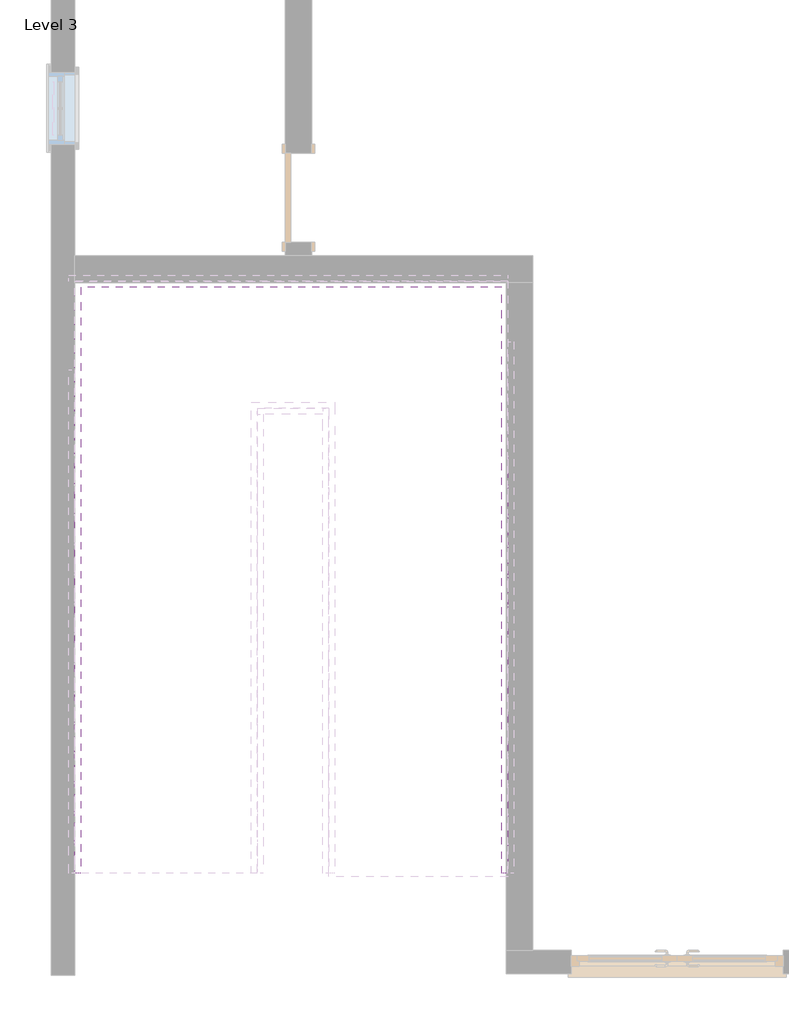
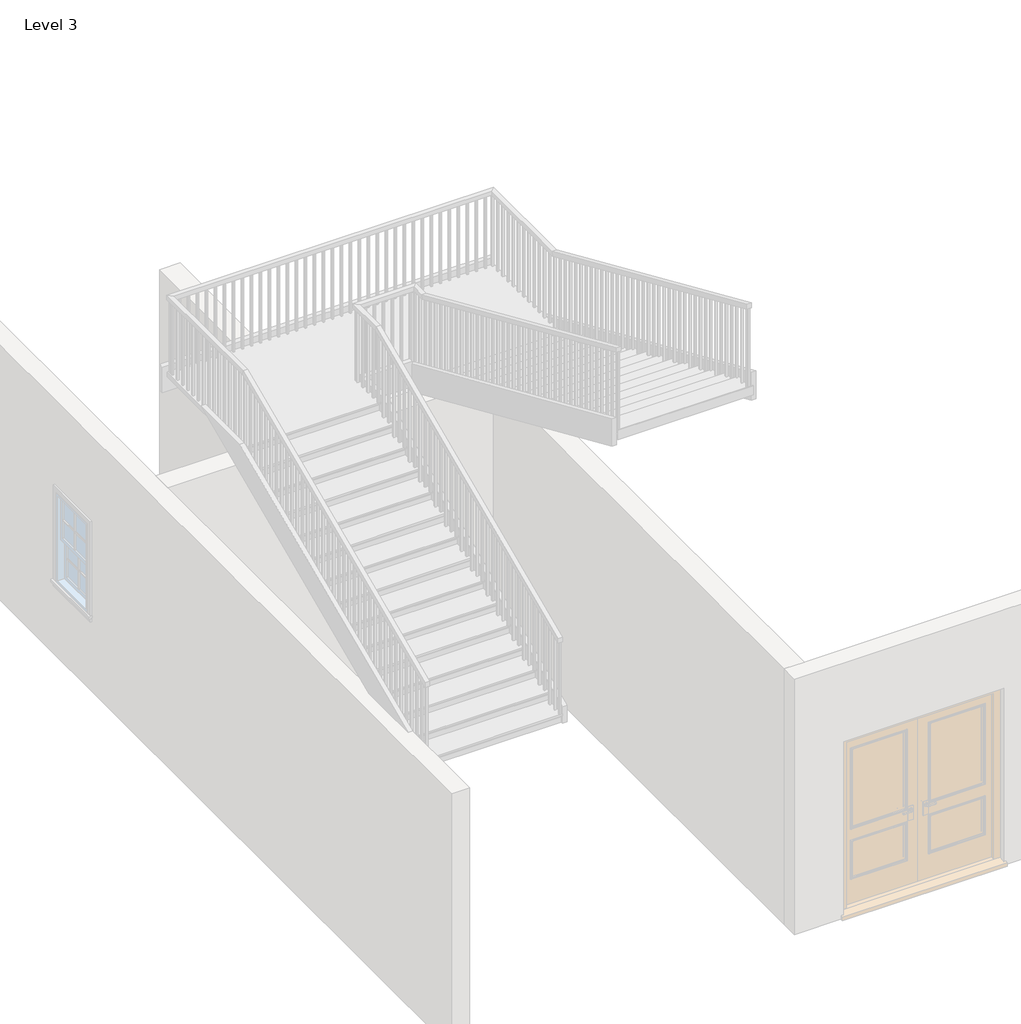
# One storey, part 5 of 6: 1 railing.
"""IFC4 building model written with IfcOpenShell, lengths in millimetres."""

from ifc_helpers import new_model, si_unit, frame, origin, place, context, project, spatial, polyline, outline, extrude, faceted_brep, element, save

model = new_model("IFC4")

# Units and contexts
model_context = context("Model", 3, world=origin())
ifc_project = project(units=[si_unit("LENGTHUNIT", "METRE", prefix="MILLI")], contexts=[model_context])

# Site, building, storey
site = spatial("IfcSite", under=ifc_project)
building = spatial("IfcBuilding", under=site)
storey = spatial("IfcBuildingStorey", under=building, Name="Level 3", Elevation=6096.0)

# Railing
placement = place(None, origin())
element("IfcRailing", 1, ObjectType="Handrail - Rectangular", at=placement, inside=storey, context=model_context, shape_type="SolidModel", body=[
    faceted_brep([(-7554.4415084, -6973.0610642, 9865.36), (-7554.4415084, -6973.0610642, 9809.8599828), (-7503.6415084, -6973.0610642, 9809.8599828), (-7503.6415084, -6973.0610642, 9865.36), (-7554.4415084, -3417.0610642, 11430.0), (-7554.4415084, -3406.3792071, 11379.2), (-7503.6415084, -3406.3792071, 11379.2), (-7503.6415084, -3417.0610642, 11430.0), (-7554.4415084, -1928.4217109, 11430.0), (-7554.4415084, -1928.4217109, 11379.2), (-7503.6415084, -1979.2217109, 11379.2), (-7503.6415084, -1979.2217109, 11430.0), (-3866.3290366, -1928.4217109, 11430.0), (-3866.3290366, -1928.4217109, 11379.2), (-3917.1290366, -1979.2217109, 11379.2), (-3917.1290366, -1979.2217109, 11430.0), (-3866.3290366, -3163.0610642, 11430.0), (-3866.3290366, -3173.7429214, 11379.2), (-3917.1290366, -3173.7429214, 11379.2), (-3917.1290366, -3163.0610642, 11430.0), (-3866.3290366, -6973.0610642, 13106.4), (-3917.1290366, -6973.0610642, 13106.4), (-3917.1290366, -6973.0610642, 13050.8999828), (-3866.3290366, -6973.0610642, 13050.8999828)], [[[0, 1, 2, 3]], [[1, 0, 4, 5]], [[2, 1, 5, 6]], [[3, 2, 6, 7]], [[0, 3, 7, 4]], [[5, 4, 8, 9]], [[6, 5, 9, 10]], [[7, 6, 10, 11]], [[4, 7, 11, 8]], [[9, 8, 12, 13]], [[10, 9, 13, 14]], [[11, 10, 14, 15]], [[8, 11, 15, 12]], [[13, 12, 16, 17]], [[14, 13, 17, 18]], [[15, 14, 18, 19]], [[12, 15, 19, 16]], [[20, 21, 22, 23]], [[17, 16, 20, 23]], [[18, 17, 23, 22]], [[19, 18, 22, 21]], [[16, 19, 21, 20]]]),
    extrude(outline(polyline([(-6922.6967109, 13028.7396674), (-6922.6967109, 12080.24), (-6941.7467109, 12080.24), (-6941.7467109, 13037.1216674), (-6922.6967109, 13028.7396674)])), frame((-3901.2540366, 0.0, 0.0), z_axis=(1.0, 0.0, 0.0), x_axis=(0.0, 1.0, 0.0)), (0.0, 0.0, 1.0), 19.05),
    extrude(outline(polyline([(-6821.0967109, 12984.0356674), (-6821.0967109, 12080.24), (-6840.1467109, 12080.24), (-6840.1467109, 12992.4176674), (-6821.0967109, 12984.0356674)])), frame((-3901.2540366, 0.0, 0.0), z_axis=(1.0, 0.0, 0.0), x_axis=(0.0, 1.0, 0.0)), (0.0, 0.0, 1.0), 19.05),
    extrude(outline(polyline([(-6719.4967109, 12939.3316674), (-6719.4967109, 12080.24), (-6738.5467109, 12080.24), (-6738.5467109, 12947.7136674), (-6719.4967109, 12939.3316674)])), frame((-3901.2540366, 0.0, 0.0), z_axis=(1.0, 0.0, 0.0), x_axis=(0.0, 1.0, 0.0)), (0.0, 0.0, 1.0), 19.05),
    extrude(outline(polyline([(-6617.8967109, 12894.6276674), (-6617.8967109, 11968.48), (-6636.9467109, 11968.48), (-6636.9467109, 12903.0096674), (-6617.8967109, 12894.6276674)])), frame((-3901.2540366, 0.0, 0.0), z_axis=(1.0, 0.0, 0.0), x_axis=(0.0, 1.0, 0.0)), (0.0, 0.0, 1.0), 19.05),
    extrude(outline(polyline([(-6516.2967109, 12849.9236674), (-6516.2967109, 11968.48), (-6535.3467109, 11968.48), (-6535.3467109, 12858.3056674), (-6516.2967109, 12849.9236674)])), frame((-3901.2540366, 0.0, 0.0), z_axis=(1.0, 0.0, 0.0), x_axis=(0.0, 1.0, 0.0)), (0.0, 0.0, 1.0), 19.05),
    extrude(outline(polyline([(-6414.6967109, 12805.2196674), (-6414.6967109, 11856.72), (-6433.7467109, 11856.72), (-6433.7467109, 12813.6016674), (-6414.6967109, 12805.2196674)])), frame((-3901.2540366, 0.0, 0.0), z_axis=(1.0, 0.0, 0.0), x_axis=(0.0, 1.0, 0.0)), (0.0, 0.0, 1.0), 19.05),
    extrude(outline(polyline([(-6313.0967109, 12760.5156674), (-6313.0967109, 11856.72), (-6332.1467109, 11856.72), (-6332.1467109, 12768.8976674), (-6313.0967109, 12760.5156674)])), frame((-3901.2540366, 0.0, 0.0), z_axis=(1.0, 0.0, 0.0), x_axis=(0.0, 1.0, 0.0)), (0.0, 0.0, 1.0), 19.05),
    extrude(outline(polyline([(-6211.4967109, 12715.8116674), (-6211.4967109, 11856.72), (-6230.5467109, 11856.72), (-6230.5467109, 12724.1936674), (-6211.4967109, 12715.8116674)])), frame((-3901.2540366, 0.0, 0.0), z_axis=(1.0, 0.0, 0.0), x_axis=(0.0, 1.0, 0.0)), (0.0, 0.0, 1.0), 19.05),
    extrude(outline(polyline([(-6109.8967109, 12671.1076674), (-6109.8967109, 11744.96), (-6128.9467109, 11744.96), (-6128.9467109, 12679.4896674), (-6109.8967109, 12671.1076674)])), frame((-3901.2540366, 0.0, 0.0), z_axis=(1.0, 0.0, 0.0), x_axis=(0.0, 1.0, 0.0)), (0.0, 0.0, 1.0), 19.05),
    extrude(outline(polyline([(-6008.2967109, 12626.4036674), (-6008.2967109, 11744.96), (-6027.3467109, 11744.96), (-6027.3467109, 12634.7856674), (-6008.2967109, 12626.4036674)])), frame((-3901.2540366, 0.0, 0.0), z_axis=(1.0, 0.0, 0.0), x_axis=(0.0, 1.0, 0.0)), (0.0, 0.0, 1.0), 19.05),
    extrude(outline(polyline([(-5906.6967109, 12581.6996674), (-5906.6967109, 11633.2), (-5925.7467109, 11633.2), (-5925.7467109, 12590.0816674), (-5906.6967109, 12581.6996674)])), frame((-3901.2540366, 0.0, 0.0), z_axis=(1.0, 0.0, 0.0), x_axis=(0.0, 1.0, 0.0)), (0.0, 0.0, 1.0), 19.05),
    extrude(outline(polyline([(-5805.0967109, 12536.9956674), (-5805.0967109, 11633.2), (-5824.1467109, 11633.2), (-5824.1467109, 12545.3776674), (-5805.0967109, 12536.9956674)])), frame((-3901.2540366, 0.0, 0.0), z_axis=(1.0, 0.0, 0.0), x_axis=(0.0, 1.0, 0.0)), (0.0, 0.0, 1.0), 19.05),
    extrude(outline(polyline([(-5703.4967109, 12492.2916674), (-5703.4967109, 11633.2), (-5722.5467109, 11633.2), (-5722.5467109, 12500.6736674), (-5703.4967109, 12492.2916674)])), frame((-3901.2540366, 0.0, 0.0), z_axis=(1.0, 0.0, 0.0), x_axis=(0.0, 1.0, 0.0)), (0.0, 0.0, 1.0), 19.05),
    extrude(outline(polyline([(-5601.8967109, 12447.5876674), (-5601.8967109, 11521.44), (-5620.9467109, 11521.44), (-5620.9467109, 12455.9696674), (-5601.8967109, 12447.5876674)])), frame((-3901.2540366, 0.0, 0.0), z_axis=(1.0, 0.0, 0.0), x_axis=(0.0, 1.0, 0.0)), (0.0, 0.0, 1.0), 19.05),
    extrude(outline(polyline([(-5500.2967109, 12402.8836674), (-5500.2967109, 11521.44), (-5519.3467109, 11521.44), (-5519.3467109, 12411.2656674), (-5500.2967109, 12402.8836674)])), frame((-3901.2540366, 0.0, 0.0), z_axis=(1.0, 0.0, 0.0), x_axis=(0.0, 1.0, 0.0)), (0.0, 0.0, 1.0), 19.05),
    extrude(outline(polyline([(-5398.6967109, 12358.1796674), (-5398.6967109, 11409.68), (-5417.7467109, 11409.68), (-5417.7467109, 12366.5616674), (-5398.6967109, 12358.1796674)])), frame((-3901.2540366, 0.0, 0.0), z_axis=(1.0, 0.0, 0.0), x_axis=(0.0, 1.0, 0.0)), (0.0, 0.0, 1.0), 19.05),
    extrude(outline(polyline([(-5297.0967109, 12313.4756674), (-5297.0967109, 11409.68), (-5316.1467109, 11409.68), (-5316.1467109, 12321.8576674), (-5297.0967109, 12313.4756674)])), frame((-3901.2540366, 0.0, 0.0), z_axis=(1.0, 0.0, 0.0), x_axis=(0.0, 1.0, 0.0)), (0.0, 0.0, 1.0), 19.05),
    extrude(outline(polyline([(-5195.4967109, 12268.7716674), (-5195.4967109, 11409.68), (-5214.5467109, 11409.68), (-5214.5467109, 12277.1536674), (-5195.4967109, 12268.7716674)])), frame((-3901.2540366, 0.0, 0.0), z_axis=(1.0, 0.0, 0.0), x_axis=(0.0, 1.0, 0.0)), (0.0, 0.0, 1.0), 19.05),
    extrude(outline(polyline([(-5093.8967109, 12224.0676674), (-5093.8967109, 11297.92), (-5112.9467109, 11297.92), (-5112.9467109, 12232.4496674), (-5093.8967109, 12224.0676674)])), frame((-3901.2540366, 0.0, 0.0), z_axis=(1.0, 0.0, 0.0), x_axis=(0.0, 1.0, 0.0)), (0.0, 0.0, 1.0), 19.05),
    extrude(outline(polyline([(-4992.2967109, 12179.3636674), (-4992.2967109, 11297.92), (-5011.3467109, 11297.92), (-5011.3467109, 12187.7456674), (-4992.2967109, 12179.3636674)])), frame((-3901.2540366, 0.0, 0.0), z_axis=(1.0, 0.0, 0.0), x_axis=(0.0, 1.0, 0.0)), (0.0, 0.0, 1.0), 19.05),
    extrude(outline(polyline([(-4890.6967109, 12134.6596674), (-4890.6967109, 11186.16), (-4909.7467109, 11186.16), (-4909.7467109, 12143.0416674), (-4890.6967109, 12134.6596674)])), frame((-3901.2540366, 0.0, 0.0), z_axis=(1.0, 0.0, 0.0), x_axis=(0.0, 1.0, 0.0)), (0.0, 0.0, 1.0), 19.05),
    extrude(outline(polyline([(-4789.0967109, 12089.9556674), (-4789.0967109, 11186.16), (-4808.1467109, 11186.16), (-4808.1467109, 12098.3376674), (-4789.0967109, 12089.9556674)])), frame((-3901.2540366, 0.0, 0.0), z_axis=(1.0, 0.0, 0.0), x_axis=(0.0, 1.0, 0.0)), (0.0, 0.0, 1.0), 19.05),
    extrude(outline(polyline([(-4687.4967109, 12045.2516674), (-4687.4967109, 11186.16), (-4706.5467109, 11186.16), (-4706.5467109, 12053.6336674), (-4687.4967109, 12045.2516674)])), frame((-3901.2540366, 0.0, 0.0), z_axis=(1.0, 0.0, 0.0), x_axis=(0.0, 1.0, 0.0)), (0.0, 0.0, 1.0), 19.05),
    extrude(outline(polyline([(-4585.8967109, 12000.5476674), (-4585.8967109, 11074.4), (-4604.9467109, 11074.4), (-4604.9467109, 12008.9296674), (-4585.8967109, 12000.5476674)])), frame((-3901.2540366, 0.0, 0.0), z_axis=(1.0, 0.0, 0.0), x_axis=(0.0, 1.0, 0.0)), (0.0, 0.0, 1.0), 19.05),
    extrude(outline(polyline([(-4484.2967109, 11955.8436674), (-4484.2967109, 11074.4), (-4503.3467109, 11074.4), (-4503.3467109, 11964.2256674), (-4484.2967109, 11955.8436674)])), frame((-3901.2540366, 0.0, 0.0), z_axis=(1.0, 0.0, 0.0), x_axis=(0.0, 1.0, 0.0)), (0.0, 0.0, 1.0), 19.05),
    extrude(outline(polyline([(-4382.6967109, 11911.1396674), (-4382.6967109, 10962.64), (-4401.7467109, 10962.64), (-4401.7467109, 11919.5216674), (-4382.6967109, 11911.1396674)])), frame((-3901.2540366, 0.0, 0.0), z_axis=(1.0, 0.0, 0.0), x_axis=(0.0, 1.0, 0.0)), (0.0, 0.0, 1.0), 19.05),
    extrude(outline(polyline([(-4281.0967109, 11866.4356674), (-4281.0967109, 10962.64), (-4300.1467109, 10962.64), (-4300.1467109, 11874.8176674), (-4281.0967109, 11866.4356674)])), frame((-3901.2540366, 0.0, 0.0), z_axis=(1.0, 0.0, 0.0), x_axis=(0.0, 1.0, 0.0)), (0.0, 0.0, 1.0), 19.05),
    extrude(outline(polyline([(-4179.4967109, 11821.7316674), (-4179.4967109, 10962.64), (-4198.5467109, 10962.64), (-4198.5467109, 11830.1136674), (-4179.4967109, 11821.7316674)])), frame((-3901.2540366, 0.0, 0.0), z_axis=(1.0, 0.0, 0.0), x_axis=(0.0, 1.0, 0.0)), (0.0, 0.0, 1.0), 19.05),
    extrude(outline(polyline([(-4077.8967109, 11777.0276674), (-4077.8967109, 10850.88), (-4096.9467109, 10850.88), (-4096.9467109, 11785.4096674), (-4077.8967109, 11777.0276674)])), frame((-3901.2540366, 0.0, 0.0), z_axis=(1.0, 0.0, 0.0), x_axis=(0.0, 1.0, 0.0)), (0.0, 0.0, 1.0), 19.05),
    extrude(outline(polyline([(-3976.2967109, 11732.3236674), (-3976.2967109, 10850.88), (-3995.3467109, 10850.88), (-3995.3467109, 11740.7056674), (-3976.2967109, 11732.3236674)])), frame((-3901.2540366, 0.0, 0.0), z_axis=(1.0, 0.0, 0.0), x_axis=(0.0, 1.0, 0.0)), (0.0, 0.0, 1.0), 19.05),
    extrude(outline(polyline([(-3874.6967109, 11687.6196674), (-3874.6967109, 10739.12), (-3893.7467109, 10739.12), (-3893.7467109, 11696.0016674), (-3874.6967109, 11687.6196674)])), frame((-3901.2540366, 0.0, 0.0), z_axis=(1.0, 0.0, 0.0), x_axis=(0.0, 1.0, 0.0)), (0.0, 0.0, 1.0), 19.05),
    extrude(outline(polyline([(-3773.0967109, 11642.9156674), (-3773.0967109, 10739.12), (-3792.1467109, 10739.12), (-3792.1467109, 11651.2976674), (-3773.0967109, 11642.9156674)])), frame((-3901.2540366, 0.0, 0.0), z_axis=(1.0, 0.0, 0.0), x_axis=(0.0, 1.0, 0.0)), (0.0, 0.0, 1.0), 19.05),
    extrude(outline(polyline([(-3671.4967109, 11598.2116674), (-3671.4967109, 10739.12), (-3690.5467109, 10739.12), (-3690.5467109, 11606.5936674), (-3671.4967109, 11598.2116674)])), frame((-3901.2540366, 0.0, 0.0), z_axis=(1.0, 0.0, 0.0), x_axis=(0.0, 1.0, 0.0)), (0.0, 0.0, 1.0), 19.05),
    extrude(outline(polyline([(-3569.8967109, 11553.5076674), (-3569.8967109, 10627.36), (-3588.9467109, 10627.36), (-3588.9467109, 11561.8896674), (-3569.8967109, 11553.5076674)])), frame((-3901.2540366, 0.0, 0.0), z_axis=(1.0, 0.0, 0.0), x_axis=(0.0, 1.0, 0.0)), (0.0, 0.0, 1.0), 19.05),
    extrude(outline(polyline([(-3468.2967109, 11508.8036674), (-3468.2967109, 10627.36), (-3487.3467109, 10627.36), (-3487.3467109, 11517.1856674), (-3468.2967109, 11508.8036674)])), frame((-3901.2540366, 0.0, 0.0), z_axis=(1.0, 0.0, 0.0), x_axis=(0.0, 1.0, 0.0)), (0.0, 0.0, 1.0), 19.05),
    extrude(outline(polyline([(-3366.6967109, 11464.0996674), (-3366.6967109, 10515.6), (-3385.7467109, 10515.6), (-3385.7467109, 11472.4816674), (-3366.6967109, 11464.0996674)])), frame((-3901.2540366, 0.0, 0.0), z_axis=(1.0, 0.0, 0.0), x_axis=(0.0, 1.0, 0.0)), (0.0, 0.0, 1.0), 19.05),
    extrude(outline(polyline([(-3265.0967109, 11419.3956674), (-3265.0967109, 10515.6), (-3284.1467109, 10515.6), (-3284.1467109, 11427.7776674), (-3265.0967109, 11419.3956674)])), frame((-3901.2540366, 0.0, 0.0), z_axis=(1.0, 0.0, 0.0), x_axis=(0.0, 1.0, 0.0)), (0.0, 0.0, 1.0), 19.05),
    extrude(outline(polyline([(-3163.4967109, 11374.6916674), (-3163.4967109, 10515.6), (-3182.5467109, 10515.6), (-3182.5467109, 11383.0736674), (-3163.4967109, 11374.6916674)])), frame((-3901.2540366, 0.0, 0.0), z_axis=(1.0, 0.0, 0.0), x_axis=(0.0, 1.0, 0.0)), (0.0, 0.0, 1.0), 19.05),
    extrude(outline(polyline([(-3882.2040366, -3061.8967109), (-3882.2040366, -3080.9467109), (-3901.2540366, -3080.9467109), (-3901.2540366, -3061.8967109), (-3882.2040366, -3061.8967109)])), frame((0.0, 0.0, 10515.6), z_axis=(0.0, 0.0, 1.0), x_axis=(1.0, 0.0, 0.0)), (0.0, 0.0, 1.0), 863.6),
    extrude(outline(polyline([(-3882.2040366, -2960.2967109), (-3882.2040366, -2979.3467109), (-3901.2540366, -2979.3467109), (-3901.2540366, -2960.2967109), (-3882.2040366, -2960.2967109)])), frame((0.0, 0.0, 10515.6), z_axis=(0.0, 0.0, 1.0), x_axis=(1.0, 0.0, 0.0)), (0.0, 0.0, 1.0), 863.6),
    extrude(outline(polyline([(-3882.2040366, -2858.6967109), (-3882.2040366, -2877.7467109), (-3901.2540366, -2877.7467109), (-3901.2540366, -2858.6967109), (-3882.2040366, -2858.6967109)])), frame((0.0, 0.0, 10515.6), z_axis=(0.0, 0.0, 1.0), x_axis=(1.0, 0.0, 0.0)), (0.0, 0.0, 1.0), 863.6),
    extrude(outline(polyline([(-3882.2040366, -2757.0967109), (-3882.2040366, -2776.1467109), (-3901.2540366, -2776.1467109), (-3901.2540366, -2757.0967109), (-3882.2040366, -2757.0967109)])), frame((0.0, 0.0, 10515.6), z_axis=(0.0, 0.0, 1.0), x_axis=(1.0, 0.0, 0.0)), (0.0, 0.0, 1.0), 863.6),
    extrude(outline(polyline([(-3882.2040366, -2655.4967109), (-3882.2040366, -2674.5467109), (-3901.2540366, -2674.5467109), (-3901.2540366, -2655.4967109), (-3882.2040366, -2655.4967109)])), frame((0.0, 0.0, 10515.6), z_axis=(0.0, 0.0, 1.0), x_axis=(1.0, 0.0, 0.0)), (0.0, 0.0, 1.0), 863.6),
    extrude(outline(polyline([(-3882.2040366, -2553.8967109), (-3882.2040366, -2572.9467109), (-3901.2540366, -2572.9467109), (-3901.2540366, -2553.8967109), (-3882.2040366, -2553.8967109)])), frame((0.0, 0.0, 10515.6), z_axis=(0.0, 0.0, 1.0), x_axis=(1.0, 0.0, 0.0)), (0.0, 0.0, 1.0), 863.6),
    extrude(outline(polyline([(-3882.2040366, -2452.2967109), (-3882.2040366, -2471.3467109), (-3901.2540366, -2471.3467109), (-3901.2540366, -2452.2967109), (-3882.2040366, -2452.2967109)])), frame((0.0, 0.0, 10515.6), z_axis=(0.0, 0.0, 1.0), x_axis=(1.0, 0.0, 0.0)), (0.0, 0.0, 1.0), 863.6),
    extrude(outline(polyline([(-3882.2040366, -2350.6967109), (-3882.2040366, -2369.7467109), (-3901.2540366, -2369.7467109), (-3901.2540366, -2350.6967109), (-3882.2040366, -2350.6967109)])), frame((0.0, 0.0, 10515.6), z_axis=(0.0, 0.0, 1.0), x_axis=(1.0, 0.0, 0.0)), (0.0, 0.0, 1.0), 863.6),
    extrude(outline(polyline([(-3882.2040366, -2249.0967109), (-3882.2040366, -2268.1467109), (-3901.2540366, -2268.1467109), (-3901.2540366, -2249.0967109), (-3882.2040366, -2249.0967109)])), frame((0.0, 0.0, 10515.6), z_axis=(0.0, 0.0, 1.0), x_axis=(1.0, 0.0, 0.0)), (0.0, 0.0, 1.0), 863.6),
    extrude(outline(polyline([(-3882.2040366, -2147.4967109), (-3882.2040366, -2166.5467109), (-3901.2540366, -2166.5467109), (-3901.2540366, -2147.4967109), (-3882.2040366, -2147.4967109)])), frame((0.0, 0.0, 10515.6), z_axis=(0.0, 0.0, 1.0), x_axis=(1.0, 0.0, 0.0)), (0.0, 0.0, 1.0), 863.6),
    extrude(outline(polyline([(-3882.2040366, -2045.8967109), (-3882.2040366, -2064.9467109), (-3901.2540366, -2064.9467109), (-3901.2540366, -2045.8967109), (-3882.2040366, -2045.8967109)])), frame((0.0, 0.0, 10515.6), z_axis=(0.0, 0.0, 1.0), x_axis=(1.0, 0.0, 0.0)), (0.0, 0.0, 1.0), 863.6),
    extrude(outline(polyline([(-3982.5665084, -1944.2967109), (-3963.5165084, -1944.2967109), (-3963.5165084, -1963.3467109), (-3982.5665084, -1963.3467109), (-3982.5665084, -1944.2967109)])), frame((0.0, 0.0, 10515.6), z_axis=(0.0, 0.0, 1.0), x_axis=(1.0, 0.0, 0.0)), (0.0, 0.0, 1.0), 863.6),
    extrude(outline(polyline([(-4084.1665084, -1944.2967109), (-4065.1165084, -1944.2967109), (-4065.1165084, -1963.3467109), (-4084.1665084, -1963.3467109), (-4084.1665084, -1944.2967109)])), frame((0.0, 0.0, 10515.6), z_axis=(0.0, 0.0, 1.0), x_axis=(1.0, 0.0, 0.0)), (0.0, 0.0, 1.0), 863.6),
    extrude(outline(polyline([(-4185.7665084, -1944.2967109), (-4166.7165084, -1944.2967109), (-4166.7165084, -1963.3467109), (-4185.7665084, -1963.3467109), (-4185.7665084, -1944.2967109)])), frame((0.0, 0.0, 10515.6), z_axis=(0.0, 0.0, 1.0), x_axis=(1.0, 0.0, 0.0)), (0.0, 0.0, 1.0), 863.6),
    extrude(outline(polyline([(-4287.3665084, -1944.2967109), (-4268.3165084, -1944.2967109), (-4268.3165084, -1963.3467109), (-4287.3665084, -1963.3467109), (-4287.3665084, -1944.2967109)])), frame((0.0, 0.0, 10515.6), z_axis=(0.0, 0.0, 1.0), x_axis=(1.0, 0.0, 0.0)), (0.0, 0.0, 1.0), 863.6),
    extrude(outline(polyline([(-4388.9665084, -1944.2967109), (-4369.9165084, -1944.2967109), (-4369.9165084, -1963.3467109), (-4388.9665084, -1963.3467109), (-4388.9665084, -1944.2967109)])), frame((0.0, 0.0, 10515.6), z_axis=(0.0, 0.0, 1.0), x_axis=(1.0, 0.0, 0.0)), (0.0, 0.0, 1.0), 863.6),
    extrude(outline(polyline([(-4490.5665084, -1944.2967109), (-4471.5165084, -1944.2967109), (-4471.5165084, -1963.3467109), (-4490.5665084, -1963.3467109), (-4490.5665084, -1944.2967109)])), frame((0.0, 0.0, 10515.6), z_axis=(0.0, 0.0, 1.0), x_axis=(1.0, 0.0, 0.0)), (0.0, 0.0, 1.0), 863.6),
    extrude(outline(polyline([(-4592.1665084, -1944.2967109), (-4573.1165084, -1944.2967109), (-4573.1165084, -1963.3467109), (-4592.1665084, -1963.3467109), (-4592.1665084, -1944.2967109)])), frame((0.0, 0.0, 10515.6), z_axis=(0.0, 0.0, 1.0), x_axis=(1.0, 0.0, 0.0)), (0.0, 0.0, 1.0), 863.6),
    extrude(outline(polyline([(-4693.7665084, -1944.2967109), (-4674.7165084, -1944.2967109), (-4674.7165084, -1963.3467109), (-4693.7665084, -1963.3467109), (-4693.7665084, -1944.2967109)])), frame((0.0, 0.0, 10515.6), z_axis=(0.0, 0.0, 1.0), x_axis=(1.0, 0.0, 0.0)), (0.0, 0.0, 1.0), 863.6),
    extrude(outline(polyline([(-4795.3665084, -1944.2967109), (-4776.3165084, -1944.2967109), (-4776.3165084, -1963.3467109), (-4795.3665084, -1963.3467109), (-4795.3665084, -1944.2967109)])), frame((0.0, 0.0, 10515.6), z_axis=(0.0, 0.0, 1.0), x_axis=(1.0, 0.0, 0.0)), (0.0, 0.0, 1.0), 863.6),
    extrude(outline(polyline([(-4896.9665084, -1944.2967109), (-4877.9165084, -1944.2967109), (-4877.9165084, -1963.3467109), (-4896.9665084, -1963.3467109), (-4896.9665084, -1944.2967109)])), frame((0.0, 0.0, 10515.6), z_axis=(0.0, 0.0, 1.0), x_axis=(1.0, 0.0, 0.0)), (0.0, 0.0, 1.0), 863.6),
    extrude(outline(polyline([(-4998.5665084, -1944.2967109), (-4979.5165084, -1944.2967109), (-4979.5165084, -1963.3467109), (-4998.5665084, -1963.3467109), (-4998.5665084, -1944.2967109)])), frame((0.0, 0.0, 10515.6), z_axis=(0.0, 0.0, 1.0), x_axis=(1.0, 0.0, 0.0)), (0.0, 0.0, 1.0), 863.6),
    extrude(outline(polyline([(-5100.1665084, -1944.2967109), (-5081.1165084, -1944.2967109), (-5081.1165084, -1963.3467109), (-5100.1665084, -1963.3467109), (-5100.1665084, -1944.2967109)])), frame((0.0, 0.0, 10515.6), z_axis=(0.0, 0.0, 1.0), x_axis=(1.0, 0.0, 0.0)), (0.0, 0.0, 1.0), 863.6),
    extrude(outline(polyline([(-5201.7665084, -1944.2967109), (-5182.7165084, -1944.2967109), (-5182.7165084, -1963.3467109), (-5201.7665084, -1963.3467109), (-5201.7665084, -1944.2967109)])), frame((0.0, 0.0, 10515.6), z_axis=(0.0, 0.0, 1.0), x_axis=(1.0, 0.0, 0.0)), (0.0, 0.0, 1.0), 863.6),
    extrude(outline(polyline([(-5303.3665084, -1944.2967109), (-5284.3165084, -1944.2967109), (-5284.3165084, -1963.3467109), (-5303.3665084, -1963.3467109), (-5303.3665084, -1944.2967109)])), frame((0.0, 0.0, 10515.6), z_axis=(0.0, 0.0, 1.0), x_axis=(1.0, 0.0, 0.0)), (0.0, 0.0, 1.0), 863.6),
    extrude(outline(polyline([(-5404.9665084, -1944.2967109), (-5385.9165084, -1944.2967109), (-5385.9165084, -1963.3467109), (-5404.9665084, -1963.3467109), (-5404.9665084, -1944.2967109)])), frame((0.0, 0.0, 10515.6), z_axis=(0.0, 0.0, 1.0), x_axis=(1.0, 0.0, 0.0)), (0.0, 0.0, 1.0), 863.6),
    extrude(outline(polyline([(-5506.5665084, -1944.2967109), (-5487.5165084, -1944.2967109), (-5487.5165084, -1963.3467109), (-5506.5665084, -1963.3467109), (-5506.5665084, -1944.2967109)])), frame((0.0, 0.0, 10515.6), z_axis=(0.0, 0.0, 1.0), x_axis=(1.0, 0.0, 0.0)), (0.0, 0.0, 1.0), 863.6),
    extrude(outline(polyline([(-5608.1665084, -1944.2967109), (-5589.1165084, -1944.2967109), (-5589.1165084, -1963.3467109), (-5608.1665084, -1963.3467109), (-5608.1665084, -1944.2967109)])), frame((0.0, 0.0, 10515.6), z_axis=(0.0, 0.0, 1.0), x_axis=(1.0, 0.0, 0.0)), (0.0, 0.0, 1.0), 863.6),
    extrude(outline(polyline([(-5709.7665084, -1944.2967109), (-5690.7165084, -1944.2967109), (-5690.7165084, -1963.3467109), (-5709.7665084, -1963.3467109), (-5709.7665084, -1944.2967109)])), frame((0.0, 0.0, 10515.6), z_axis=(0.0, 0.0, 1.0), x_axis=(1.0, 0.0, 0.0)), (0.0, 0.0, 1.0), 863.6),
    extrude(outline(polyline([(-5811.3665084, -1944.2967109), (-5792.3165084, -1944.2967109), (-5792.3165084, -1963.3467109), (-5811.3665084, -1963.3467109), (-5811.3665084, -1944.2967109)])), frame((0.0, 0.0, 10515.6), z_axis=(0.0, 0.0, 1.0), x_axis=(1.0, 0.0, 0.0)), (0.0, 0.0, 1.0), 863.6),
    extrude(outline(polyline([(-5912.9665084, -1944.2967109), (-5893.9165084, -1944.2967109), (-5893.9165084, -1963.3467109), (-5912.9665084, -1963.3467109), (-5912.9665084, -1944.2967109)])), frame((0.0, 0.0, 10515.6), z_axis=(0.0, 0.0, 1.0), x_axis=(1.0, 0.0, 0.0)), (0.0, 0.0, 1.0), 863.6),
    extrude(outline(polyline([(-6014.5665084, -1944.2967109), (-5995.5165084, -1944.2967109), (-5995.5165084, -1963.3467109), (-6014.5665084, -1963.3467109), (-6014.5665084, -1944.2967109)])), frame((0.0, 0.0, 10515.6), z_axis=(0.0, 0.0, 1.0), x_axis=(1.0, 0.0, 0.0)), (0.0, 0.0, 1.0), 863.6),
    extrude(outline(polyline([(-6116.1665084, -1944.2967109), (-6097.1165084, -1944.2967109), (-6097.1165084, -1963.3467109), (-6116.1665084, -1963.3467109), (-6116.1665084, -1944.2967109)])), frame((0.0, 0.0, 10515.6), z_axis=(0.0, 0.0, 1.0), x_axis=(1.0, 0.0, 0.0)), (0.0, 0.0, 1.0), 863.6),
    extrude(outline(polyline([(-6217.7665084, -1944.2967109), (-6198.7165084, -1944.2967109), (-6198.7165084, -1963.3467109), (-6217.7665084, -1963.3467109), (-6217.7665084, -1944.2967109)])), frame((0.0, 0.0, 10515.6), z_axis=(0.0, 0.0, 1.0), x_axis=(1.0, 0.0, 0.0)), (0.0, 0.0, 1.0), 863.6),
    extrude(outline(polyline([(-6319.3665084, -1944.2967109), (-6300.3165084, -1944.2967109), (-6300.3165084, -1963.3467109), (-6319.3665084, -1963.3467109), (-6319.3665084, -1944.2967109)])), frame((0.0, 0.0, 10515.6), z_axis=(0.0, 0.0, 1.0), x_axis=(1.0, 0.0, 0.0)), (0.0, 0.0, 1.0), 863.6),
    extrude(outline(polyline([(-6420.9665084, -1944.2967109), (-6401.9165084, -1944.2967109), (-6401.9165084, -1963.3467109), (-6420.9665084, -1963.3467109), (-6420.9665084, -1944.2967109)])), frame((0.0, 0.0, 10515.6), z_axis=(0.0, 0.0, 1.0), x_axis=(1.0, 0.0, 0.0)), (0.0, 0.0, 1.0), 863.6),
    extrude(outline(polyline([(-6522.5665084, -1944.2967109), (-6503.5165084, -1944.2967109), (-6503.5165084, -1963.3467109), (-6522.5665084, -1963.3467109), (-6522.5665084, -1944.2967109)])), frame((0.0, 0.0, 10515.6), z_axis=(0.0, 0.0, 1.0), x_axis=(1.0, 0.0, 0.0)), (0.0, 0.0, 1.0), 863.6),
    extrude(outline(polyline([(-6624.1665084, -1944.2967109), (-6605.1165084, -1944.2967109), (-6605.1165084, -1963.3467109), (-6624.1665084, -1963.3467109), (-6624.1665084, -1944.2967109)])), frame((0.0, 0.0, 10515.6), z_axis=(0.0, 0.0, 1.0), x_axis=(1.0, 0.0, 0.0)), (0.0, 0.0, 1.0), 863.6),
    extrude(outline(polyline([(-6725.7665084, -1944.2967109), (-6706.7165084, -1944.2967109), (-6706.7165084, -1963.3467109), (-6725.7665084, -1963.3467109), (-6725.7665084, -1944.2967109)])), frame((0.0, 0.0, 10515.6), z_axis=(0.0, 0.0, 1.0), x_axis=(1.0, 0.0, 0.0)), (0.0, 0.0, 1.0), 863.6),
    extrude(outline(polyline([(-6827.3665084, -1944.2967109), (-6808.3165084, -1944.2967109), (-6808.3165084, -1963.3467109), (-6827.3665084, -1963.3467109), (-6827.3665084, -1944.2967109)])), frame((0.0, 0.0, 10515.6), z_axis=(0.0, 0.0, 1.0), x_axis=(1.0, 0.0, 0.0)), (0.0, 0.0, 1.0), 863.6),
    extrude(outline(polyline([(-6928.9665084, -1944.2967109), (-6909.9165084, -1944.2967109), (-6909.9165084, -1963.3467109), (-6928.9665084, -1963.3467109), (-6928.9665084, -1944.2967109)])), frame((0.0, 0.0, 10515.6), z_axis=(0.0, 0.0, 1.0), x_axis=(1.0, 0.0, 0.0)), (0.0, 0.0, 1.0), 863.6),
    extrude(outline(polyline([(-7030.5665084, -1944.2967109), (-7011.5165084, -1944.2967109), (-7011.5165084, -1963.3467109), (-7030.5665084, -1963.3467109), (-7030.5665084, -1944.2967109)])), frame((0.0, 0.0, 10515.6), z_axis=(0.0, 0.0, 1.0), x_axis=(1.0, 0.0, 0.0)), (0.0, 0.0, 1.0), 863.6),
    extrude(outline(polyline([(-7132.1665084, -1944.2967109), (-7113.1165084, -1944.2967109), (-7113.1165084, -1963.3467109), (-7132.1665084, -1963.3467109), (-7132.1665084, -1944.2967109)])), frame((0.0, 0.0, 10515.6), z_axis=(0.0, 0.0, 1.0), x_axis=(1.0, 0.0, 0.0)), (0.0, 0.0, 1.0), 863.6),
    extrude(outline(polyline([(-7233.7665084, -1944.2967109), (-7214.7165084, -1944.2967109), (-7214.7165084, -1963.3467109), (-7233.7665084, -1963.3467109), (-7233.7665084, -1944.2967109)])), frame((0.0, 0.0, 10515.6), z_axis=(0.0, 0.0, 1.0), x_axis=(1.0, 0.0, 0.0)), (0.0, 0.0, 1.0), 863.6),
    extrude(outline(polyline([(-7335.3665084, -1944.2967109), (-7316.3165084, -1944.2967109), (-7316.3165084, -1963.3467109), (-7335.3665084, -1963.3467109), (-7335.3665084, -1944.2967109)])), frame((0.0, 0.0, 10515.6), z_axis=(0.0, 0.0, 1.0), x_axis=(1.0, 0.0, 0.0)), (0.0, 0.0, 1.0), 863.6),
    extrude(outline(polyline([(-7436.9665084, -1944.2967109), (-7417.9165084, -1944.2967109), (-7417.9165084, -1963.3467109), (-7436.9665084, -1963.3467109), (-7436.9665084, -1944.2967109)])), frame((0.0, 0.0, 10515.6), z_axis=(0.0, 0.0, 1.0), x_axis=(1.0, 0.0, 0.0)), (0.0, 0.0, 1.0), 863.6),
    extrude(outline(polyline([(-7538.5665084, -2004.1860642), (-7538.5665084, -1985.1360642), (-7519.5165084, -1985.1360642), (-7519.5165084, -2004.1860642), (-7538.5665084, -2004.1860642)])), frame((0.0, 0.0, 10515.6), z_axis=(0.0, 0.0, 1.0), x_axis=(1.0, 0.0, 0.0)), (0.0, 0.0, 1.0), 863.6),
    extrude(outline(polyline([(-7538.5665084, -2105.7860642), (-7538.5665084, -2086.7360642), (-7519.5165084, -2086.7360642), (-7519.5165084, -2105.7860642), (-7538.5665084, -2105.7860642)])), frame((0.0, 0.0, 10515.6), z_axis=(0.0, 0.0, 1.0), x_axis=(1.0, 0.0, 0.0)), (0.0, 0.0, 1.0), 863.6),
    extrude(outline(polyline([(-7538.5665084, -2207.3860642), (-7538.5665084, -2188.3360642), (-7519.5165084, -2188.3360642), (-7519.5165084, -2207.3860642), (-7538.5665084, -2207.3860642)])), frame((0.0, 0.0, 10515.6), z_axis=(0.0, 0.0, 1.0), x_axis=(1.0, 0.0, 0.0)), (0.0, 0.0, 1.0), 863.6),
    extrude(outline(polyline([(-7538.5665084, -2308.9860642), (-7538.5665084, -2289.9360642), (-7519.5165084, -2289.9360642), (-7519.5165084, -2308.9860642), (-7538.5665084, -2308.9860642)])), frame((0.0, 0.0, 10515.6), z_axis=(0.0, 0.0, 1.0), x_axis=(1.0, 0.0, 0.0)), (0.0, 0.0, 1.0), 863.6),
    extrude(outline(polyline([(-7538.5665084, -2410.5860642), (-7538.5665084, -2391.5360642), (-7519.5165084, -2391.5360642), (-7519.5165084, -2410.5860642), (-7538.5665084, -2410.5860642)])), frame((0.0, 0.0, 10515.6), z_axis=(0.0, 0.0, 1.0), x_axis=(1.0, 0.0, 0.0)), (0.0, 0.0, 1.0), 863.6),
    extrude(outline(polyline([(-7538.5665084, -2512.1860642), (-7538.5665084, -2493.1360642), (-7519.5165084, -2493.1360642), (-7519.5165084, -2512.1860642), (-7538.5665084, -2512.1860642)])), frame((0.0, 0.0, 10515.6), z_axis=(0.0, 0.0, 1.0), x_axis=(1.0, 0.0, 0.0)), (0.0, 0.0, 1.0), 863.6),
    extrude(outline(polyline([(-7538.5665084, -2613.7860642), (-7538.5665084, -2594.7360642), (-7519.5165084, -2594.7360642), (-7519.5165084, -2613.7860642), (-7538.5665084, -2613.7860642)])), frame((0.0, 0.0, 10515.6), z_axis=(0.0, 0.0, 1.0), x_axis=(1.0, 0.0, 0.0)), (0.0, 0.0, 1.0), 863.6),
    extrude(outline(polyline([(-7538.5665084, -2715.3860642), (-7538.5665084, -2696.3360642), (-7519.5165084, -2696.3360642), (-7519.5165084, -2715.3860642), (-7538.5665084, -2715.3860642)])), frame((0.0, 0.0, 10515.6), z_axis=(0.0, 0.0, 1.0), x_axis=(1.0, 0.0, 0.0)), (0.0, 0.0, 1.0), 863.6),
    extrude(outline(polyline([(-7538.5665084, -2816.9860642), (-7538.5665084, -2797.9360642), (-7519.5165084, -2797.9360642), (-7519.5165084, -2816.9860642), (-7538.5665084, -2816.9860642)])), frame((0.0, 0.0, 10515.6), z_axis=(0.0, 0.0, 1.0), x_axis=(1.0, 0.0, 0.0)), (0.0, 0.0, 1.0), 863.6),
    extrude(outline(polyline([(-7538.5665084, -2918.5860642), (-7538.5665084, -2899.5360642), (-7519.5165084, -2899.5360642), (-7519.5165084, -2918.5860642), (-7538.5665084, -2918.5860642)])), frame((0.0, 0.0, 10515.6), z_axis=(0.0, 0.0, 1.0), x_axis=(1.0, 0.0, 0.0)), (0.0, 0.0, 1.0), 863.6),
    extrude(outline(polyline([(-7538.5665084, -3020.1860642), (-7538.5665084, -3001.1360642), (-7519.5165084, -3001.1360642), (-7519.5165084, -3020.1860642), (-7538.5665084, -3020.1860642)])), frame((0.0, 0.0, 10515.6), z_axis=(0.0, 0.0, 1.0), x_axis=(1.0, 0.0, 0.0)), (0.0, 0.0, 1.0), 863.6),
    extrude(outline(polyline([(-7538.5665084, -3121.7860642), (-7538.5665084, -3102.7360642), (-7519.5165084, -3102.7360642), (-7519.5165084, -3121.7860642), (-7538.5665084, -3121.7860642)])), frame((0.0, 0.0, 10515.6), z_axis=(0.0, 0.0, 1.0), x_axis=(1.0, 0.0, 0.0)), (0.0, 0.0, 1.0), 863.6),
    extrude(outline(polyline([(-7538.5665084, -3223.3860642), (-7538.5665084, -3204.3360642), (-7519.5165084, -3204.3360642), (-7519.5165084, -3223.3860642), (-7538.5665084, -3223.3860642)])), frame((0.0, 0.0, 10515.6), z_axis=(0.0, 0.0, 1.0), x_axis=(1.0, 0.0, 0.0)), (0.0, 0.0, 1.0), 863.6),
    extrude(outline(polyline([(-7538.5665084, -3324.9860642), (-7538.5665084, -3305.9360642), (-7519.5165084, -3305.9360642), (-7519.5165084, -3324.9860642), (-7538.5665084, -3324.9860642)])), frame((0.0, 0.0, 10515.6), z_axis=(0.0, 0.0, 1.0), x_axis=(1.0, 0.0, 0.0)), (0.0, 0.0, 1.0), 863.6),
    extrude(outline(polyline([(-3407.5360642, 11378.6909828), (-3407.5360642, 10515.6), (-3426.5860642, 10515.6), (-3426.5860642, 11370.3089828), (-3407.5360642, 11378.6909828)])), frame((-7538.5665084, 0.0, 0.0), z_axis=(1.0, 0.0, 0.0), x_axis=(0.0, 1.0, 0.0)), (0.0, 0.0, 1.0), 19.05),
    extrude(outline(polyline([(-3509.1360642, 11333.9869828), (-3509.1360642, 10403.84), (-3528.1860642, 10403.84), (-3528.1860642, 11325.6049828), (-3509.1360642, 11333.9869828)])), frame((-7538.5665084, 0.0, 0.0), z_axis=(1.0, 0.0, 0.0), x_axis=(0.0, 1.0, 0.0)), (0.0, 0.0, 1.0), 19.05),
    extrude(outline(polyline([(-3610.7360642, 11289.2829828), (-3610.7360642, 10403.84), (-3629.7860642, 10403.84), (-3629.7860642, 11280.9009828), (-3610.7360642, 11289.2829828)])), frame((-7538.5665084, 0.0, 0.0), z_axis=(1.0, 0.0, 0.0), x_axis=(0.0, 1.0, 0.0)), (0.0, 0.0, 1.0), 19.05),
    extrude(outline(polyline([(-3712.3360642, 11244.5789828), (-3712.3360642, 10292.08), (-3731.3860642, 10292.08), (-3731.3860642, 11236.1969828), (-3712.3360642, 11244.5789828)])), frame((-7538.5665084, 0.0, 0.0), z_axis=(1.0, 0.0, 0.0), x_axis=(0.0, 1.0, 0.0)), (0.0, 0.0, 1.0), 19.05),
    extrude(outline(polyline([(-3813.9360642, 11199.8749828), (-3813.9360642, 10292.08), (-3832.9860642, 10292.08), (-3832.9860642, 11191.4929828), (-3813.9360642, 11199.8749828)])), frame((-7538.5665084, 0.0, 0.0), z_axis=(1.0, 0.0, 0.0), x_axis=(0.0, 1.0, 0.0)), (0.0, 0.0, 1.0), 19.05),
    extrude(outline(polyline([(-3915.5360642, 11155.1709828), (-3915.5360642, 10292.08), (-3934.5860642, 10292.08), (-3934.5860642, 11146.7889828), (-3915.5360642, 11155.1709828)])), frame((-7538.5665084, 0.0, 0.0), z_axis=(1.0, 0.0, 0.0), x_axis=(0.0, 1.0, 0.0)), (0.0, 0.0, 1.0), 19.05),
    extrude(outline(polyline([(-4017.1360642, 11110.4669828), (-4017.1360642, 10180.32), (-4036.1860642, 10180.32), (-4036.1860642, 11102.0849828), (-4017.1360642, 11110.4669828)])), frame((-7538.5665084, 0.0, 0.0), z_axis=(1.0, 0.0, 0.0), x_axis=(0.0, 1.0, 0.0)), (0.0, 0.0, 1.0), 19.05),
    extrude(outline(polyline([(-4118.7360642, 11065.7629828), (-4118.7360642, 10180.32), (-4137.7860642, 10180.32), (-4137.7860642, 11057.3809828), (-4118.7360642, 11065.7629828)])), frame((-7538.5665084, 0.0, 0.0), z_axis=(1.0, 0.0, 0.0), x_axis=(0.0, 1.0, 0.0)), (0.0, 0.0, 1.0), 19.05),
    extrude(outline(polyline([(-4220.3360642, 11021.0589828), (-4220.3360642, 10068.56), (-4239.3860642, 10068.56), (-4239.3860642, 11012.6769828), (-4220.3360642, 11021.0589828)])), frame((-7538.5665084, 0.0, 0.0), z_axis=(1.0, 0.0, 0.0), x_axis=(0.0, 1.0, 0.0)), (0.0, 0.0, 1.0), 19.05),
    extrude(outline(polyline([(-4321.9360642, 10976.3549828), (-4321.9360642, 10068.56), (-4340.9860642, 10068.56), (-4340.9860642, 10967.9729828), (-4321.9360642, 10976.3549828)])), frame((-7538.5665084, 0.0, 0.0), z_axis=(1.0, 0.0, 0.0), x_axis=(0.0, 1.0, 0.0)), (0.0, 0.0, 1.0), 19.05),
    extrude(outline(polyline([(-4423.5360642, 10931.6509828), (-4423.5360642, 10068.56), (-4442.5860642, 10068.56), (-4442.5860642, 10923.2689828), (-4423.5360642, 10931.6509828)])), frame((-7538.5665084, 0.0, 0.0), z_axis=(1.0, 0.0, 0.0), x_axis=(0.0, 1.0, 0.0)), (0.0, 0.0, 1.0), 19.05),
    extrude(outline(polyline([(-4525.1360642, 10886.9469828), (-4525.1360642, 9956.8), (-4544.1860642, 9956.8), (-4544.1860642, 10878.5649828), (-4525.1360642, 10886.9469828)])), frame((-7538.5665084, 0.0, 0.0), z_axis=(1.0, 0.0, 0.0), x_axis=(0.0, 1.0, 0.0)), (0.0, 0.0, 1.0), 19.05),
    extrude(outline(polyline([(-4626.7360642, 10842.2429828), (-4626.7360642, 9956.8), (-4645.7860642, 9956.8), (-4645.7860642, 10833.8609828), (-4626.7360642, 10842.2429828)])), frame((-7538.5665084, 0.0, 0.0), z_axis=(1.0, 0.0, 0.0), x_axis=(0.0, 1.0, 0.0)), (0.0, 0.0, 1.0), 19.05),
    extrude(outline(polyline([(-4728.3360642, 10797.5389828), (-4728.3360642, 9845.04), (-4747.3860642, 9845.04), (-4747.3860642, 10789.1569828), (-4728.3360642, 10797.5389828)])), frame((-7538.5665084, 0.0, 0.0), z_axis=(1.0, 0.0, 0.0), x_axis=(0.0, 1.0, 0.0)), (0.0, 0.0, 1.0), 19.05),
    extrude(outline(polyline([(-4829.9360642, 10752.8349828), (-4829.9360642, 9845.04), (-4848.9860642, 9845.04), (-4848.9860642, 10744.4529828), (-4829.9360642, 10752.8349828)])), frame((-7538.5665084, 0.0, 0.0), z_axis=(1.0, 0.0, 0.0), x_axis=(0.0, 1.0, 0.0)), (0.0, 0.0, 1.0), 19.05),
    extrude(outline(polyline([(-4931.5360642, 10708.1309828), (-4931.5360642, 9845.04), (-4950.5860642, 9845.04), (-4950.5860642, 10699.7489828), (-4931.5360642, 10708.1309828)])), frame((-7538.5665084, 0.0, 0.0), z_axis=(1.0, 0.0, 0.0), x_axis=(0.0, 1.0, 0.0)), (0.0, 0.0, 1.0), 19.05),
    extrude(outline(polyline([(-5033.1360642, 10663.4269828), (-5033.1360642, 9733.28), (-5052.1860642, 9733.28), (-5052.1860642, 10655.0449828), (-5033.1360642, 10663.4269828)])), frame((-7538.5665084, 0.0, 0.0), z_axis=(1.0, 0.0, 0.0), x_axis=(0.0, 1.0, 0.0)), (0.0, 0.0, 1.0), 19.05),
    extrude(outline(polyline([(-5134.7360642, 10618.7229828), (-5134.7360642, 9733.28), (-5153.7860642, 9733.28), (-5153.7860642, 10610.3409828), (-5134.7360642, 10618.7229828)])), frame((-7538.5665084, 0.0, 0.0), z_axis=(1.0, 0.0, 0.0), x_axis=(0.0, 1.0, 0.0)), (0.0, 0.0, 1.0), 19.05),
    extrude(outline(polyline([(-5236.3360642, 10574.0189828), (-5236.3360642, 9621.52), (-5255.3860642, 9621.52), (-5255.3860642, 10565.6369828), (-5236.3360642, 10574.0189828)])), frame((-7538.5665084, 0.0, 0.0), z_axis=(1.0, 0.0, 0.0), x_axis=(0.0, 1.0, 0.0)), (0.0, 0.0, 1.0), 19.05),
    extrude(outline(polyline([(-5337.9360642, 10529.3149828), (-5337.9360642, 9621.52), (-5356.9860642, 9621.52), (-5356.9860642, 10520.9329828), (-5337.9360642, 10529.3149828)])), frame((-7538.5665084, 0.0, 0.0), z_axis=(1.0, 0.0, 0.0), x_axis=(0.0, 1.0, 0.0)), (0.0, 0.0, 1.0), 19.05),
    extrude(outline(polyline([(-5439.5360642, 10484.6109828), (-5439.5360642, 9621.52), (-5458.5860642, 9621.52), (-5458.5860642, 10476.2289828), (-5439.5360642, 10484.6109828)])), frame((-7538.5665084, 0.0, 0.0), z_axis=(1.0, 0.0, 0.0), x_axis=(0.0, 1.0, 0.0)), (0.0, 0.0, 1.0), 19.05),
    extrude(outline(polyline([(-5541.1360642, 10439.9069828), (-5541.1360642, 9509.76), (-5560.1860642, 9509.76), (-5560.1860642, 10431.5249828), (-5541.1360642, 10439.9069828)])), frame((-7538.5665084, 0.0, 0.0), z_axis=(1.0, 0.0, 0.0), x_axis=(0.0, 1.0, 0.0)), (0.0, 0.0, 1.0), 19.05),
    extrude(outline(polyline([(-5642.7360642, 10395.2029828), (-5642.7360642, 9509.76), (-5661.7860642, 9509.76), (-5661.7860642, 10386.8209828), (-5642.7360642, 10395.2029828)])), frame((-7538.5665084, 0.0, 0.0), z_axis=(1.0, 0.0, 0.0), x_axis=(0.0, 1.0, 0.0)), (0.0, 0.0, 1.0), 19.05),
    extrude(outline(polyline([(-5744.3360642, 10350.4989828), (-5744.3360642, 9398.0), (-5763.3860642, 9398.0), (-5763.3860642, 10342.1169828), (-5744.3360642, 10350.4989828)])), frame((-7538.5665084, 0.0, 0.0), z_axis=(1.0, 0.0, 0.0), x_axis=(0.0, 1.0, 0.0)), (0.0, 0.0, 1.0), 19.05),
    extrude(outline(polyline([(-5845.9360642, 10305.7949828), (-5845.9360642, 9398.0), (-5864.9860642, 9398.0), (-5864.9860642, 10297.4129828), (-5845.9360642, 10305.7949828)])), frame((-7538.5665084, 0.0, 0.0), z_axis=(1.0, 0.0, 0.0), x_axis=(0.0, 1.0, 0.0)), (0.0, 0.0, 1.0), 19.05),
    extrude(outline(polyline([(-5947.5360642, 10261.0909828), (-5947.5360642, 9398.0), (-5966.5860642, 9398.0), (-5966.5860642, 10252.7089828), (-5947.5360642, 10261.0909828)])), frame((-7538.5665084, 0.0, 0.0), z_axis=(1.0, 0.0, 0.0), x_axis=(0.0, 1.0, 0.0)), (0.0, 0.0, 1.0), 19.05),
    extrude(outline(polyline([(-6049.1360642, 10216.3869828), (-6049.1360642, 9286.24), (-6068.1860642, 9286.24), (-6068.1860642, 10208.0049828), (-6049.1360642, 10216.3869828)])), frame((-7538.5665084, 0.0, 0.0), z_axis=(1.0, 0.0, 0.0), x_axis=(0.0, 1.0, 0.0)), (0.0, 0.0, 1.0), 19.05),
    extrude(outline(polyline([(-6150.7360642, 10171.6829828), (-6150.7360642, 9286.24), (-6169.7860642, 9286.24), (-6169.7860642, 10163.3009828), (-6150.7360642, 10171.6829828)])), frame((-7538.5665084, 0.0, 0.0), z_axis=(1.0, 0.0, 0.0), x_axis=(0.0, 1.0, 0.0)), (0.0, 0.0, 1.0), 19.05),
    extrude(outline(polyline([(-6252.3360642, 10126.9789828), (-6252.3360642, 9174.48), (-6271.3860642, 9174.48), (-6271.3860642, 10118.5969828), (-6252.3360642, 10126.9789828)])), frame((-7538.5665084, 0.0, 0.0), z_axis=(1.0, 0.0, 0.0), x_axis=(0.0, 1.0, 0.0)), (0.0, 0.0, 1.0), 19.05),
    extrude(outline(polyline([(-6353.9360642, 10082.2749828), (-6353.9360642, 9174.48), (-6372.9860642, 9174.48), (-6372.9860642, 10073.8929828), (-6353.9360642, 10082.2749828)])), frame((-7538.5665084, 0.0, 0.0), z_axis=(1.0, 0.0, 0.0), x_axis=(0.0, 1.0, 0.0)), (0.0, 0.0, 1.0), 19.05),
    extrude(outline(polyline([(-6455.5360642, 10037.5709828), (-6455.5360642, 9174.48), (-6474.5860642, 9174.48), (-6474.5860642, 10029.1889828), (-6455.5360642, 10037.5709828)])), frame((-7538.5665084, 0.0, 0.0), z_axis=(1.0, 0.0, 0.0), x_axis=(0.0, 1.0, 0.0)), (0.0, 0.0, 1.0), 19.05),
    extrude(outline(polyline([(-6557.1360642, 9992.8669828), (-6557.1360642, 9062.72), (-6576.1860642, 9062.72), (-6576.1860642, 9984.4849828), (-6557.1360642, 9992.8669828)])), frame((-7538.5665084, 0.0, 0.0), z_axis=(1.0, 0.0, 0.0), x_axis=(0.0, 1.0, 0.0)), (0.0, 0.0, 1.0), 19.05),
    extrude(outline(polyline([(-6658.7360642, 9948.1629828), (-6658.7360642, 9062.72), (-6677.7860642, 9062.72), (-6677.7860642, 9939.7809828), (-6658.7360642, 9948.1629828)])), frame((-7538.5665084, 0.0, 0.0), z_axis=(1.0, 0.0, 0.0), x_axis=(0.0, 1.0, 0.0)), (0.0, 0.0, 1.0), 19.05),
    extrude(outline(polyline([(-6760.3360642, 9903.4589828), (-6760.3360642, 8950.96), (-6779.3860642, 8950.96), (-6779.3860642, 9895.0769828), (-6760.3360642, 9903.4589828)])), frame((-7538.5665084, 0.0, 0.0), z_axis=(1.0, 0.0, 0.0), x_axis=(0.0, 1.0, 0.0)), (0.0, 0.0, 1.0), 19.05),
    extrude(outline(polyline([(-6861.9360642, 9858.7549828), (-6861.9360642, 8950.96), (-6880.9860642, 8950.96), (-6880.9860642, 9850.3729828), (-6861.9360642, 9858.7549828)])), frame((-7538.5665084, 0.0, 0.0), z_axis=(1.0, 0.0, 0.0), x_axis=(0.0, 1.0, 0.0)), (0.0, 0.0, 1.0), 19.05),
    extrude(outline(polyline([(-3901.2540366, -1944.2967109), (-3882.2040366, -1944.2967109), (-3882.2040366, -1963.3467109), (-3901.2540366, -1963.3467109), (-3901.2540366, -1944.2967109)])), frame((0.0, 0.0, 10515.6), z_axis=(0.0, 0.0, 1.0), x_axis=(1.0, 0.0, 0.0)), (0.0, 0.0, 1.0), 863.6),
    extrude(outline(polyline([(-7538.5665084, -1963.3467109), (-7538.5665084, -1944.2967109), (-7519.5165084, -1944.2967109), (-7519.5165084, -1963.3467109), (-7538.5665084, -1963.3467109)])), frame((0.0, 0.0, 10515.6), z_axis=(0.0, 0.0, 1.0), x_axis=(1.0, 0.0, 0.0)), (0.0, 0.0, 1.0), 863.6),
    extrude(outline(polyline([(-6954.0110642, 13042.5179828), (-6954.0110642, 12080.24), (-6973.0610642, 12080.24), (-6973.0610642, 13050.8999828), (-6954.0110642, 13042.5179828)])), frame((-3901.2540366, 0.0, 0.0), z_axis=(1.0, 0.0, 0.0), x_axis=(0.0, 1.0, 0.0)), (0.0, 0.0, 1.0), 19.05),
    extrude(outline(polyline([(-6954.0110642, 9818.2419828), (-6954.0110642, 8950.96), (-6973.0610642, 8950.96), (-6973.0610642, 9809.8599828), (-6954.0110642, 9818.2419828)])), frame((-7538.5665084, 0.0, 0.0), z_axis=(1.0, 0.0, 0.0), x_axis=(0.0, 1.0, 0.0)), (0.0, 0.0, 1.0), 19.05),
])

save(model, "model.ifc")

# Revit data of these elements
# Type "Handrail - Rectangular"
#   Assembly Code = "C2010400"
#   built-in parameter 1008612 = 0.0416667 (stored number, unit not read)
#   built-in parameter 1008611 = 0.0416667 (stored number, unit not read)
#   built-in parameter 1008609 = 0.333333 (stored number, unit not read)
#   built-in parameter 1008604 = 0.166667 (stored number, unit not read)
#   built-in parameter 1008603 = 0.166667 (stored number, unit not read)
#   Railing Height = 3' - 0"
#   built-in parameter 1008630 = 2
#   built-in parameter 1008610 = 2
#   built-in parameter 1008618 = Baluster - Square : 3/4"
# Element 1 (IfcRailing, "Handrail - Rectangular")
#   Phase Created = New Construction
